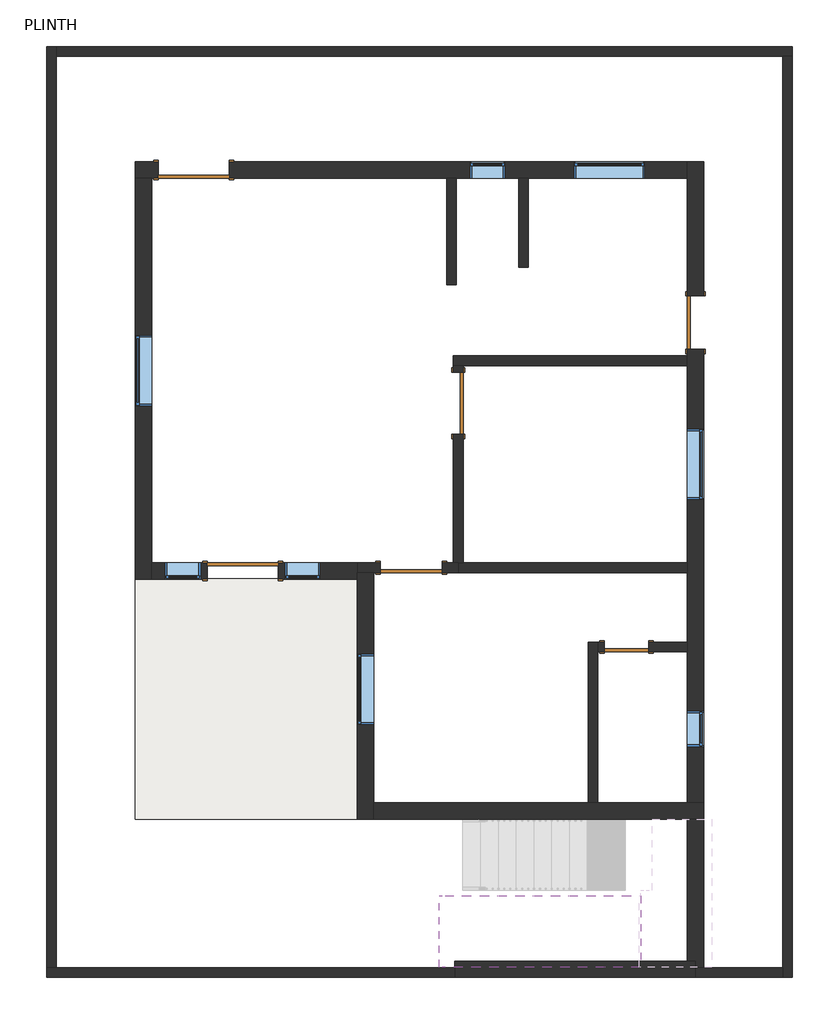
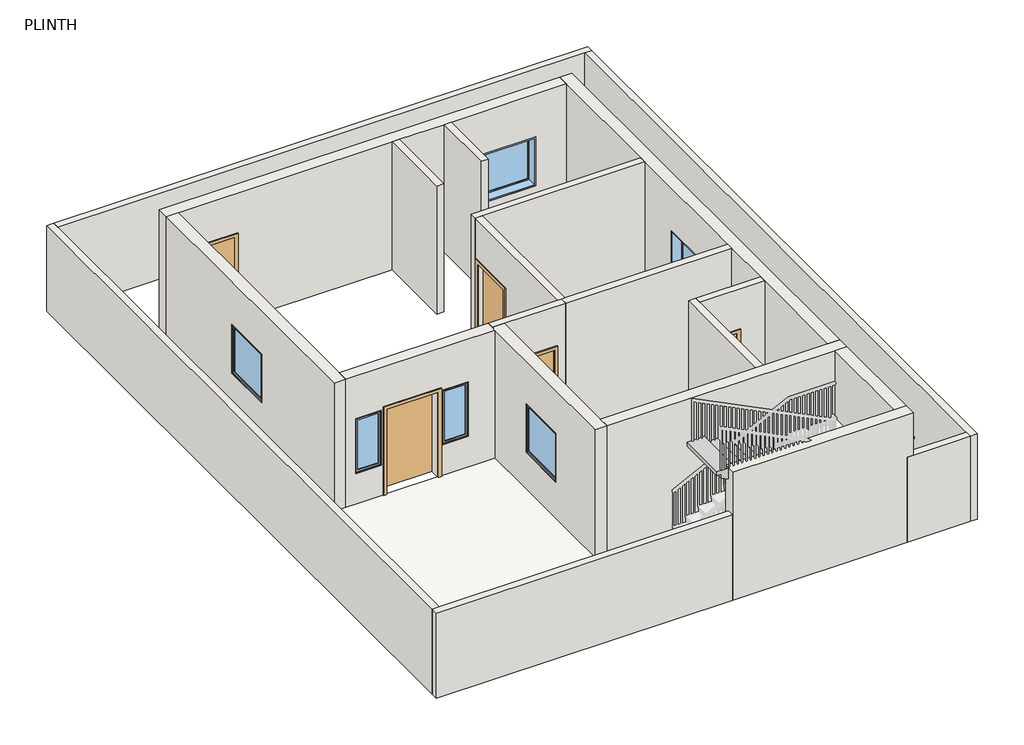
# One storey, part 1 of 3: 21 walls, 8 windows, 6 doors, 1 slab, 1 stair flight.
"""IFC4 building model written with IfcOpenShell, lengths in millimetres."""

from ifc_helpers import new_model, si_unit, frame, origin, origin_with_axes, place, context, project, spatial, polyline, outline, extrude, faceted_brep, transform, mapped, element, save
from components import door_9181f8a1, door_11d56761, door_bd8f54db, single_flush_3_x7_4f727f60, single_flush_4_x7_4e2c9459, single_flush_4_x7_d8936398, fixed_2_x2_ad5176ef, fixed_2_x4_5_07468de1, fixed_4_x4_67ff7140

model = new_model("IFC4")

# Units and contexts
model_context = context("Model", 3, world=origin())
ifc_project = project(units=[si_unit("LENGTHUNIT", "METRE", prefix="MILLI")], contexts=[model_context])

# Site, building, storey
site = spatial("IfcSite", under=ifc_project)
building = spatial("IfcBuilding", under=site)
storey = spatial("IfcBuildingStorey", under=building, Name="PLINTH", Elevation=0.0)

# Doors
placement = place(None, origin())
door_shape = door_9181f8a1(model_context)
element("IfcDoor", 1, ObjectType="Single-Flush : 2'6\"X7' 2", at=placement, inside=storey, context=model_context, shape_type="MappedRepresentation", body=[
    mapped(door_shape, transform((-10460.62252, 168.0193844, 0.0), x_axis=(-1.0, 0.0, 0.0), y_axis=(0.0, -1.0, 0.0), z_axis=(0.0, 0.0, 1.0))),
])
door_2_shape = door_11d56761(model_context)
element("IfcDoor", 2, ObjectType="Single-Flush : 3'6\"X7'", at=placement, inside=storey, context=model_context, shape_type="MappedRepresentation", body=[
    mapped(door_2_shape, transform((-14155.62252, 1526.2193844, 0.0), x_axis=(-1.0, 0.0, 0.0), y_axis=(0.0, -1.0, 0.0), z_axis=(0.0, 0.0, 1.0))),
])
door_3_shape = door_bd8f54db(model_context)
element("IfcDoor", 3, ObjectType="Single-Flush : 3'6\"X7'", at=placement, inside=storey, context=model_context, shape_type="MappedRepresentation", body=[
    mapped(door_3_shape, transform((-13348.82252, 4348.8193844, 0.0), x_axis=(0.0, 1.0, 0.0), y_axis=(-1.0, 0.0, 0.0), z_axis=(0.0, 0.0, 1.0))),
])
single_flush_3_x7_shape = single_flush_3_x7_4f727f60(model_context)
element("IfcDoor", 4, ObjectType="Single-Flush : 3'X7'", at=placement, inside=storey, context=model_context, shape_type="MappedRepresentation", body=[
    mapped(single_flush_3_x7_shape, transform((-9278.12252, 5733.8193844, 0.0), x_axis=(0.0, -1.0, 0.0), y_axis=(1.0, 0.0, 0.0), z_axis=(0.0, 0.0, 1.0))),
])
single_flush_4_x7_shape = single_flush_4_x7_4e2c9459(model_context)
element("IfcDoor", 5, ObjectType="Single-Flush : 4'X7'", at=placement, inside=storey, context=model_context, shape_type="MappedRepresentation", body=[
    mapped(single_flush_4_x7_shape, transform((-17886.62252, 8350.7193844, 0.0), x_axis=(-1.0, 0.0, 0.0), y_axis=(0.0, -1.0, 0.0), z_axis=(0.0, 0.0, 1.0))),
])
single_flush_4_x7_2_shape = single_flush_4_x7_d8936398(model_context)
element("IfcDoor", 6, ObjectType="Single-Flush : 4'X7'", at=placement, inside=storey, context=model_context, shape_type="MappedRepresentation", body=[
    mapped(single_flush_4_x7_2_shape, transform((-17048.42252, 1468.7193844, 0.0), x_axis=(-1.0, 0.0, 0.0), y_axis=(0.0, -1.0, 0.0), z_axis=(0.0, 0.0, 1.0))),
])

# Slab
element("IfcSlab", 7, ObjectType="Generic - 12\"", at=placement, inside=storey, context=model_context, shape_type="SweptSolid", body=[
    extrude(outline(polyline([(-15084.12252, 1341.7193844), (-15084.12252, -2786.4806156), (-18891.32252, -2786.4806156), (-18891.32252, 1341.7193844), (-15084.12252, 1341.7193844)])), frame((0.0, 0.0, -609.6), z_axis=(0.0, 0.0, 1.0), x_axis=(1.0, 0.0, 0.0)), (0.0, 0.0, 1.0), 609.6),
])

# Stair flight
element("IfcStairFlight", 8, ObjectType="3/4\" Nosing 6 1/2\" Depth", at=placement, inside=storey, context=model_context, shape_type="Brep", body=[
    faceted_brep([(-10219.32252, -4107.2806156, 1676.4), (-10219.32252, -5326.4806156, 1676.4), (-10238.37252, -5326.4806156, 1524.0), (-10238.37252, -4107.2806156, 1524.0), (-10543.17252, -4107.2806156, 1676.4), (-10543.17252, -5326.4806156, 1676.4), (-10543.17252, -5326.4806156, 1491.8125885), (-10238.37252, -5326.4806156, 1339.4125885), (-10238.37252, -4107.2806156, 1339.4125885), (-10543.17252, -4107.2806156, 1491.8125885), (-10524.12252, -5326.4806156, 1828.8), (-10524.12252, -4107.2806156, 1828.8), (-10847.97252, -4107.2806156, 1828.8), (-10847.97252, -5326.4806156, 1828.8), (-10847.97252, -5326.4806156, 1644.2125885), (-10847.97252, -4107.2806156, 1644.2125885), (-10828.92252, -5326.4806156, 1981.2), (-10828.92252, -4107.2806156, 1981.2), (-11152.77252, -4107.2806156, 1981.2), (-11152.77252, -5326.4806156, 1981.2), (-11152.77252, -5326.4806156, 1796.6125885), (-11152.77252, -4107.2806156, 1796.6125885), (-11133.72252, -5326.4806156, 2133.6), (-11133.72252, -4107.2806156, 2133.6), (-11457.57252, -4107.2806156, 2133.6), (-11457.57252, -5326.4806156, 2133.6), (-11457.57252, -5326.4806156, 1949.0125885), (-11457.57252, -4107.2806156, 1949.0125885), (-11438.52252, -5326.4806156, 2286.0), (-11438.52252, -4107.2806156, 2286.0), (-11762.37252, -4107.2806156, 2286.0), (-11762.37252, -5326.4806156, 2286.0), (-11762.37252, -5326.4806156, 2101.4125885), (-11762.37252, -4107.2806156, 2101.4125885), (-11743.32252, -5326.4806156, 2438.4), (-11743.32252, -4107.2806156, 2438.4), (-12067.17252, -4107.2806156, 2438.4), (-12067.17252, -5326.4806156, 2438.4), (-12067.17252, -5326.4806156, 2253.8125885), (-12067.17252, -4107.2806156, 2253.8125885), (-12048.12252, -5326.4806156, 2590.8), (-12048.12252, -4107.2806156, 2590.8), (-12371.97252, -4107.2806156, 2590.8), (-12371.97252, -5326.4806156, 2590.8), (-12371.97252, -5326.4806156, 2406.2125885), (-12371.97252, -4107.2806156, 2406.2125885), (-12352.92252, -5326.4806156, 2743.2), (-12352.92252, -4107.2806156, 2743.2), (-12676.77252, -4107.2806156, 2743.2), (-12676.77252, -5326.4806156, 2743.2), (-12676.77252, -5326.4806156, 2558.6125885), (-12676.77252, -4107.2806156, 2558.6125885), (-12657.72252, -5326.4806156, 2895.6), (-12657.72252, -4107.2806156, 2895.6), (-12981.57252, -4107.2806156, 2895.6), (-12981.57252, -5326.4806156, 2895.6), (-12981.57252, -5326.4806156, 2711.0125885), (-12981.57252, -4107.2806156, 2711.0125885), (-12962.52252, -5326.4806156, 3048.0), (-12962.52252, -4107.2806156, 3048.0), (-13286.37252, -4107.2806156, 3048.0), (-13286.37252, -5326.4806156, 3048.0), (-13286.37252, -5326.4806156, 2863.4125885), (-13286.37252, -4107.2806156, 2863.4125885), (-13267.32252, -5326.4806156, 3200.4), (-13267.32252, -4107.2806156, 3200.4), (-13673.72252, -4107.2806156, 3200.4), (-13673.72252, -5326.4806156, 3200.4), (-13673.72252, -5326.4806156, 3098.8), (-13572.12252, -5326.4806156, 3098.8), (-13572.12252, -5326.4806156, 3006.2875885), (-13572.12252, -4107.2806156, 3006.2875885), (-13572.12252, -4107.2806156, 3098.8), (-13673.72252, -4107.2806156, 3098.8)], [[[0, 1, 2, 3]], [[1, 0, 4, 5]], [[1, 5, 6, 7, 2]], [[3, 2, 7, 8]], [[4, 0, 3, 8, 9]], [[10, 11, 12, 13]], [[10, 13, 14, 6, 5]], [[12, 11, 4, 9, 15]], [[11, 10, 5, 4]], [[16, 17, 18, 19]], [[16, 19, 20, 14, 13]], [[18, 17, 12, 15, 21]], [[17, 16, 13, 12]], [[22, 23, 24, 25]], [[22, 25, 26, 20, 19]], [[24, 23, 18, 21, 27]], [[23, 22, 19, 18]], [[28, 29, 30, 31]], [[28, 31, 32, 26, 25]], [[30, 29, 24, 27, 33]], [[29, 28, 25, 24]], [[34, 35, 36, 37]], [[34, 37, 38, 32, 31]], [[36, 35, 30, 33, 39]], [[35, 34, 31, 30]], [[40, 41, 42, 43]], [[40, 43, 44, 38, 37]], [[42, 41, 36, 39, 45]], [[41, 40, 37, 36]], [[46, 47, 48, 49]], [[46, 49, 50, 44, 43]], [[48, 47, 42, 45, 51]], [[47, 46, 43, 42]], [[52, 53, 54, 55]], [[52, 55, 56, 50, 49]], [[54, 53, 48, 51, 57]], [[53, 52, 49, 48]], [[58, 59, 60, 61]], [[58, 61, 62, 56, 55]], [[60, 59, 54, 57, 63]], [[59, 58, 55, 54]], [[64, 65, 66, 67]], [[64, 67, 68, 69, 70, 62, 61]], [[66, 65, 60, 63, 71, 72, 73]], [[71, 70, 69, 72]], [[65, 64, 61, 60]], [[7, 6, 14, 20, 26, 32, 38, 44, 50, 56, 62, 70, 71, 63, 57, 51, 45, 39, 33, 27, 21, 15, 9, 8]], [[73, 72, 69, 68]], [[73, 68, 67, 66]]]),
])

# Walls
element("IfcWall", 9, ObjectType="4.5\" WALL", at=placement, inside=storey, context=model_context, shape_type="Brep", body=[
    faceted_brep([(-13431.72252, 4996.5193844, 0.0), (-13265.92252, 4996.5193844, 0.0), (-9418.52252, 4996.5193844, 0.0), (-9418.52252, 4996.5193844, 3200.4), (-13265.92252, 4996.5193844, 3200.4), (-13431.72252, 4996.5193844, 3200.4), (-13431.72252, 5162.3193844, 0.0), (-13431.72252, 5162.3193844, 3200.4), (-9418.52252, 5162.3193844, 3200.4), (-9418.52252, 5162.3193844, 0.0)], [[[0, 1, 2, 3, 4, 5]], [[6, 7, 8, 9]], [[2, 1, 0, 6, 9]], [[5, 4, 3, 8, 7]], [[3, 2, 9, 8]], [[0, 5, 7, 6]]]),
])
element("IfcWall", 10, ObjectType="4.5\" WALL", at=placement, inside=storey, context=model_context, shape_type="SweptSolid", body=[
    extrude(outline(polyline([(-13546.72252, 6381.5193844), (-13546.72252, 8210.3193844), (-13380.92252, 8210.3193844), (-13380.92252, 6381.5193844), (-13546.72252, 6381.5193844)])), origin_with_axes(), (0.0, 0.0, 1.0), 3200.4),
])
element("IfcWall", 11, ObjectType="4.5\" WALL", at=placement, inside=storey, context=model_context, shape_type="Brep", body=[
    faceted_brep([(-9418.52252, 1609.1193844, 0.0), (-13265.92252, 1609.1193844, 0.0), (-13348.82252, 1609.1193844, 0.0), (-13348.82252, 1609.1193844, 3200.4), (-13265.92252, 1609.1193844, 3200.4), (-9418.52252, 1609.1193844, 3200.4), (-9418.52252, 1443.3193844, 0.0), (-9418.52252, 1443.3193844, 3200.4), (-13348.82252, 1443.3193844, 3200.4), (-13348.82252, 1443.3193844, 0.0)], [[[0, 1, 2, 3, 4, 5]], [[6, 7, 8, 9]], [[2, 1, 0, 6, 9]], [[3, 2, 9, 8]], [[5, 4, 3, 8, 7]], [[0, 5, 7, 6]]]),
])
element("IfcWall", 12, ObjectType="4.5\" WALL", at=placement, inside=storey, context=model_context, shape_type="SweptSolid", body=[
    extrude(outline(polyline([(-12314.12252, 6686.3193844), (-12314.12252, 8210.3193844), (-12148.32252, 8210.3193844), (-12148.32252, 6686.3193844), (-12314.12252, 6686.3193844)])), origin_with_axes(), (0.0, 0.0, 1.0), 3200.4),
])
element("IfcWall", 13, ObjectType="4.5\" WALL", at=placement, inside=storey, context=model_context, shape_type="Brep", body=[
    faceted_brep([(-14689.02252, 1609.1193844, 2133.6), (-14689.02252, 1609.1193844, 0.0), (-15084.12252, 1609.1193844, 0.0), (-15084.12252, 1609.1193844, 3200.4), (-13431.72252, 1609.1193844, 3200.4), (-13348.82252, 1609.1193844, 3200.4), (-13348.82252, 1609.1193844, 0.0), (-13431.72252, 1609.1193844, 0.0), (-13622.22252, 1609.1193844, 0.0), (-13622.22252, 1609.1193844, 2133.6), (-15084.12252, 1443.3193844, 0.0), (-14803.32252, 1443.3193844, 0.0), (-14689.02252, 1443.3193844, 0.0), (-14689.02252, 1443.3193844, 2133.6), (-13622.22252, 1443.3193844, 2133.6), (-13622.22252, 1443.3193844, 0.0), (-13348.82252, 1443.3193844, 0.0), (-13348.82252, 1443.3193844, 3200.4), (-14803.32252, 1443.3193844, 3200.4), (-15084.12252, 1443.3193844, 3200.4)], [[[0, 1, 2, 3, 4, 5, 6, 7, 8, 9]], [[10, 11, 12, 13, 14, 15, 16, 17, 18, 19]], [[2, 1, 12, 11, 10]], [[8, 7, 6, 16, 15]], [[5, 4, 3, 19, 18, 17]], [[6, 5, 17, 16]], [[3, 2, 10, 19]], [[13, 12, 1, 0]], [[14, 13, 0, 9]], [[15, 14, 9, 8]]]),
])
element("IfcWall", 14, ObjectType="4.5\" WALL", at=placement, inside=storey, context=model_context, shape_type="Brep", body=[
    faceted_brep([(-13431.72252, 1609.1193844, 3200.4), (-13431.72252, 4996.5193844, 3200.4), (-13431.72252, 4996.5193844, 0.0), (-13431.72252, 4882.2193844, 0.0), (-13431.72252, 4882.2193844, 2133.6), (-13431.72252, 3815.4193844, 2133.6), (-13431.72252, 3815.4193844, 0.0), (-13431.72252, 1609.1193844, 0.0), (-13265.92252, 4996.5193844, 3200.4), (-13265.92252, 1609.1193844, 3200.4), (-13265.92252, 1609.1193844, 0.0), (-13265.92252, 3815.4193844, 0.0), (-13265.92252, 3815.4193844, 2133.6), (-13265.92252, 4882.2193844, 2133.6), (-13265.92252, 4882.2193844, 0.0), (-13265.92252, 4996.5193844, 0.0), (-13348.82252, 1609.1193844, 0.0), (-13348.82252, 1609.1193844, 3200.4)], [[[0, 1, 2, 3, 4, 5, 6, 7]], [[8, 9, 10, 11, 12, 13, 14, 15]], [[2, 15, 14, 3]], [[10, 16, 7, 6, 11]], [[1, 0, 17, 9, 8]], [[2, 1, 8, 15]], [[0, 7, 16, 10, 9, 17]], [[13, 4, 3, 14]], [[4, 13, 12, 5]], [[5, 12, 11, 6]]]),
])
element("IfcWall", 15, ObjectType="4.5\" WALL", at=placement, inside=storey, context=model_context, shape_type="Brep", body=[
    faceted_brep([(-11121.72252, 250.9193844, 0.0), (-11121.72252, -2505.6806156, 0.0), (-11121.72252, -2505.6806156, 3200.4), (-11121.72252, 250.9193844, 3200.4), (-10955.92252, 250.9193844, 0.0), (-10955.92252, 250.9193844, 3200.4), (-10955.92252, 85.1193844, 3200.4), (-10955.92252, -2505.6806156, 3200.4), (-10955.92252, -2505.6806156, 0.0), (-10955.92252, 85.1193844, 0.0)], [[[0, 1, 2, 3]], [[4, 5, 6, 7, 8, 9]], [[1, 0, 4, 9, 8]], [[3, 2, 7, 6, 5]], [[0, 3, 5, 4]], [[2, 1, 8, 7]]]),
])
element("IfcWall", 16, ObjectType="4.5\" WALL", at=placement, inside=storey, context=model_context, shape_type="SweptSolid", body=[
    extrude(outline(polyline([(3200.4, -9418.52252), (3200.4, -10955.92252), (0.0, -10955.92252), (0.0, -10841.62252), (2133.6, -10841.62252), (2133.6, -10079.62252), (0.0, -10079.62252), (0.0, -9418.52252), (3200.4, -9418.52252)])), frame((0.0, 85.1193844, 0.0), z_axis=(0.0, 1.0, 0.0), x_axis=(0.0, 0.0, 1.0)), (0.0, 0.0, 1.0), 165.8),
])
element("IfcWall", 17, ObjectType="9\" WALL", at=placement, inside=storey, context=model_context, shape_type="Brep", body=[
    faceted_brep([(-18891.32252, 8210.3193844, 0.0), (-18610.52252, 8210.3193844, 0.0), (-18496.22252, 8210.3193844, 0.0), (-18496.22252, 8210.3193844, 2133.6), (-17277.02252, 8210.3193844, 2133.6), (-17277.02252, 8210.3193844, 0.0), (-13546.72252, 8210.3193844, 0.0), (-13380.92252, 8210.3193844, 0.0), (-12314.12252, 8210.3193844, 0.0), (-12148.32252, 8210.3193844, 0.0), (-9418.52252, 8210.3193844, 0.0), (-9418.52252, 8210.3193844, 3200.4), (-12148.32252, 8210.3193844, 3200.4), (-12314.12252, 8210.3193844, 3200.4), (-13380.92252, 8210.3193844, 3200.4), (-13546.72252, 8210.3193844, 3200.4), (-18610.52252, 8210.3193844, 3200.4), (-18891.32252, 8210.3193844, 3200.4), (-10145.07252, 8210.3193844, 2133.6), (-10145.07252, 8210.3193844, 914.4), (-11364.27252, 8210.3193844, 914.4), (-11364.27252, 8210.3193844, 2133.6), (-12542.72252, 8210.3193844, 1524.0), (-12542.72252, 8210.3193844, 914.4), (-13152.32252, 8210.3193844, 914.4), (-13152.32252, 8210.3193844, 1524.0), (-18496.22252, 8491.1193844, 2133.6), (-18496.22252, 8491.1193844, 0.0), (-18891.32252, 8491.1193844, 0.0), (-18891.32252, 8491.1193844, 3200.4), (-9418.52252, 8491.1193844, 3200.4), (-9418.52252, 8491.1193844, 0.0), (-17277.02252, 8491.1193844, 0.0), (-17277.02252, 8491.1193844, 2133.6), (-10145.07252, 8491.1193844, 2133.6), (-11364.27252, 8491.1193844, 2133.6), (-11364.27252, 8491.1193844, 914.4), (-10145.07252, 8491.1193844, 914.4), (-12542.72252, 8491.1193844, 1524.0), (-13152.32252, 8491.1193844, 1524.0), (-13152.32252, 8491.1193844, 914.4), (-12542.72252, 8491.1193844, 914.4)], [[[0, 1, 2, 3, 4, 5, 6, 7, 8, 9, 10, 11, 12, 13, 14, 15, 16, 17], [18, 19, 20, 21], [22, 23, 24, 25]], [[26, 27, 28, 29, 30, 31, 32, 33], [34, 35, 36, 37], [38, 39, 40, 41]], [[32, 31, 10, 9, 8, 7, 6, 5]], [[28, 27, 2, 1, 0]], [[17, 16, 15, 14, 13, 12, 11, 30, 29]], [[0, 17, 29, 28]], [[11, 10, 31, 30]], [[3, 2, 27, 26]], [[4, 3, 26, 33]], [[5, 4, 33, 32]], [[19, 18, 34, 37]], [[20, 19, 37, 36]], [[21, 20, 36, 35]], [[18, 21, 35, 34]], [[23, 22, 38, 41]], [[24, 23, 41, 40]], [[25, 24, 40, 39]], [[22, 25, 39, 38]]]),
])
element("IfcWall", 18, ObjectType="9\" WALL", at=placement, inside=storey, context=model_context, shape_type="Brep", body=[
    faceted_brep([(-18610.52252, 1328.3193844, 0.0), (-18610.52252, 1609.1193844, 0.0), (-18610.52252, 8210.3193844, 0.0), (-18610.52252, 8210.3193844, 3200.4), (-18610.52252, 1609.1193844, 3200.4), (-18610.52252, 1328.3193844, 3200.4), (-18610.52252, 5519.3193844, 2133.6), (-18610.52252, 5519.3193844, 914.4), (-18610.52252, 4300.1193844, 914.4), (-18610.52252, 4300.1193844, 2133.6), (-18891.32252, 1328.3193844, 0.0), (-18891.32252, 1328.3193844, 3200.4), (-18891.32252, 8210.3193844, 3200.4), (-18891.32252, 8210.3193844, 0.0), (-18891.32252, 5519.3193844, 2133.6), (-18891.32252, 4300.1193844, 2133.6), (-18891.32252, 4300.1193844, 914.4), (-18891.32252, 5519.3193844, 914.4)], [[[0, 1, 2, 3, 4, 5], [6, 7, 8, 9]], [[10, 11, 12, 13], [14, 15, 16, 17]], [[2, 1, 0, 10, 13]], [[5, 4, 3, 12, 11]], [[3, 2, 13, 12]], [[0, 5, 11, 10]], [[7, 6, 14, 17]], [[8, 7, 17, 16]], [[9, 8, 16, 15]], [[6, 9, 15, 14]]]),
])
element("IfcWall", 19, ObjectType="9\" WALL", at=placement, inside=storey, context=model_context, shape_type="Brep", body=[
    faceted_brep([(-9137.72252, -2505.6806156, 0.0), (-9418.52252, -2505.6806156, 0.0), (-10955.92252, -2505.6806156, 0.0), (-11121.72252, -2505.6806156, 0.0), (-14803.32252, -2505.6806156, 0.0), (-14803.32252, -2505.6806156, 3200.4), (-11121.72252, -2505.6806156, 3200.4), (-10955.92252, -2505.6806156, 3200.4), (-9418.52252, -2505.6806156, 3200.4), (-9137.72252, -2505.6806156, 3200.4), (-9137.72252, -2786.4806156, 0.0), (-9137.72252, -2786.4806156, 3200.4), (-9418.52252, -2786.4806156, 3200.4), (-14803.32252, -2786.4806156, 3200.4), (-14803.32252, -2786.4806156, 0.0), (-9418.52252, -2786.4806156, 0.0)], [[[0, 1, 2, 3, 4, 5, 6, 7, 8, 9]], [[10, 11, 12, 13, 14, 15]], [[4, 3, 2, 1, 0, 10, 15, 14]], [[9, 8, 7, 6, 5, 13, 12, 11]], [[0, 9, 11, 10]], [[5, 4, 14, 13]]]),
])
element("IfcWall", 20, ObjectType="9\" WALL", at=placement, inside=storey, context=model_context, shape_type="Brep", body=[
    faceted_brep([(-9418.52252, 5276.6193844, 2133.6), (-9418.52252, 5276.6193844, 0.0), (-9418.52252, 5162.3193844, 0.0), (-9418.52252, 4996.5193844, 0.0), (-9418.52252, 1609.1193844, 0.0), (-9418.52252, 1443.3193844, 0.0), (-9418.52252, 250.9193844, 0.0), (-9418.52252, 85.1193844, 0.0), (-9418.52252, -2505.6806156, 0.0), (-9418.52252, -2505.6806156, 3200.4), (-9418.52252, 85.1193844, 3200.4), (-9418.52252, 250.9193844, 3200.4), (-9418.52252, 1443.3193844, 3200.4), (-9418.52252, 1609.1193844, 3200.4), (-9418.52252, 4996.5193844, 3200.4), (-9418.52252, 5162.3193844, 3200.4), (-9418.52252, 8210.3193844, 3200.4), (-9418.52252, 8491.1193844, 3200.4), (-9418.52252, 8491.1193844, 0.0), (-9418.52252, 8210.3193844, 0.0), (-9418.52252, 6191.0193844, 0.0), (-9418.52252, 6191.0193844, 2133.6), (-9418.52252, 2693.2193844, 2133.6), (-9418.52252, 2693.2193844, 914.4), (-9418.52252, 3912.4193844, 914.4), (-9418.52252, 3912.4193844, 2133.6), (-9418.52252, -1543.8306156, 1524.0), (-9418.52252, -1543.8306156, 914.4), (-9418.52252, -934.2306156, 914.4), (-9418.52252, -934.2306156, 1524.0), (-9137.72252, -2505.6806156, 0.0), (-9137.72252, 5276.6193844, 0.0), (-9137.72252, 5276.6193844, 2133.6), (-9137.72252, 6191.0193844, 2133.6), (-9137.72252, 6191.0193844, 0.0), (-9137.72252, 8491.1193844, 0.0), (-9137.72252, 8491.1193844, 3200.4), (-9137.72252, -2505.6806156, 3200.4), (-9137.72252, 2693.2193844, 2133.6), (-9137.72252, 3912.4193844, 2133.6), (-9137.72252, 3912.4193844, 914.4), (-9137.72252, 2693.2193844, 914.4), (-9137.72252, -1543.8306156, 1524.0), (-9137.72252, -934.2306156, 1524.0), (-9137.72252, -934.2306156, 914.4), (-9137.72252, -1543.8306156, 914.4)], [[[0, 1, 2, 3, 4, 5, 6, 7, 8, 9, 10, 11, 12, 13, 14, 15, 16, 17, 18, 19, 20, 21], [22, 23, 24, 25], [26, 27, 28, 29]], [[30, 31, 32, 33, 34, 35, 36, 37], [38, 39, 40, 41], [42, 43, 44, 45]], [[20, 19, 18, 35, 34]], [[8, 7, 6, 5, 4, 3, 2, 1, 31, 30]], [[17, 16, 15, 14, 13, 12, 11, 10, 9, 37, 36]], [[18, 17, 36, 35]], [[9, 8, 30, 37]], [[23, 22, 38, 41]], [[24, 23, 41, 40]], [[25, 24, 40, 39]], [[22, 25, 39, 38]], [[32, 31, 1, 0]], [[33, 32, 0, 21]], [[34, 33, 21, 20]], [[27, 26, 42, 45]], [[28, 27, 45, 44]], [[29, 28, 44, 43]], [[26, 29, 43, 42]]]),
])
element("IfcWall", 21, ObjectType="9\" WALL", at=placement, inside=storey, context=model_context, shape_type="Brep", body=[
    faceted_brep([(-15084.12252, 1443.3193844, 0.0), (-15084.12252, 1328.3193844, 0.0), (-15084.12252, -2786.4806156, 0.0), (-15084.12252, -2786.4806156, 3200.4), (-15084.12252, 1328.3193844, 3200.4), (-15084.12252, 1443.3193844, 3200.4), (-15084.12252, 49.6693844, 2133.6), (-15084.12252, -1169.5306156, 2133.6), (-15084.12252, -1169.5306156, 914.4), (-15084.12252, 49.6693844, 914.4), (-14803.32252, 1443.3193844, 0.0), (-14803.32252, 1443.3193844, 3200.4), (-14803.32252, -2505.6806156, 3200.4), (-14803.32252, -2786.4806156, 3200.4), (-14803.32252, -2786.4806156, 0.0), (-14803.32252, -2505.6806156, 0.0), (-14803.32252, 49.6693844, 2133.6), (-14803.32252, 49.6693844, 914.4), (-14803.32252, -1169.5306156, 914.4), (-14803.32252, -1169.5306156, 2133.6)], [[[0, 1, 2, 3, 4, 5], [6, 7, 8, 9]], [[10, 11, 12, 13, 14, 15], [16, 17, 18, 19]], [[2, 1, 0, 10, 15, 14]], [[5, 4, 3, 13, 12, 11]], [[3, 2, 14, 13]], [[0, 5, 11, 10]], [[17, 16, 6, 9]], [[18, 17, 9, 8]], [[19, 18, 8, 7]], [[16, 19, 7, 6]]]),
])
element("IfcWall", 22, ObjectType="9\" WALL", at=placement, inside=storey, context=model_context, shape_type="Brep", body=[
    faceted_brep([(-17658.02252, 1609.1193844, 2133.6), (-17658.02252, 1609.1193844, 0.0), (-18610.52252, 1609.1193844, 0.0), (-18610.52252, 1609.1193844, 3200.4), (-15084.12252, 1609.1193844, 3200.4), (-15084.12252, 1609.1193844, 0.0), (-16438.82252, 1609.1193844, 0.0), (-16438.82252, 1609.1193844, 2133.6), (-16322.831064, 1609.1193844, 2133.6), (-16322.831064, 1609.1193844, 762.0), (-15713.231064, 1609.1193844, 762.0), (-15713.231064, 1609.1193844, 2133.6), (-18381.92252, 1609.1193844, 2133.6), (-18381.92252, 1609.1193844, 762.0), (-17772.32252, 1609.1193844, 762.0), (-17772.32252, 1609.1193844, 2133.6), (-18610.52252, 1328.3193844, 0.0), (-17658.02252, 1328.3193844, 0.0), (-17658.02252, 1328.3193844, 2133.6), (-16438.82252, 1328.3193844, 2133.6), (-16438.82252, 1328.3193844, 0.0), (-15084.12252, 1328.3193844, 0.0), (-15084.12252, 1328.3193844, 3200.4), (-18610.52252, 1328.3193844, 3200.4), (-16322.831064, 1328.3193844, 2133.6), (-15713.231064, 1328.3193844, 2133.6), (-15713.231064, 1328.3193844, 762.0), (-16322.831064, 1328.3193844, 762.0), (-18381.92252, 1328.3193844, 2133.6), (-17772.32252, 1328.3193844, 2133.6), (-17772.32252, 1328.3193844, 762.0), (-18381.92252, 1328.3193844, 762.0), (-15084.12252, 1443.3193844, 0.0), (-15084.12252, 1443.3193844, 3200.4)], [[[0, 1, 2, 3, 4, 5, 6, 7], [8, 9, 10, 11], [12, 13, 14, 15]], [[16, 17, 18, 19, 20, 21, 22, 23], [24, 25, 26, 27], [28, 29, 30, 31]], [[6, 5, 32, 21, 20]], [[2, 1, 17, 16]], [[4, 3, 23, 22, 33]], [[3, 2, 16, 23]], [[5, 4, 33, 22, 21, 32]], [[18, 17, 1, 0]], [[19, 18, 0, 7]], [[20, 19, 7, 6]], [[9, 8, 24, 27]], [[10, 9, 27, 26]], [[11, 10, 26, 25]], [[8, 11, 25, 24]], [[13, 12, 28, 31]], [[14, 13, 31, 30]], [[15, 14, 30, 29]], [[12, 15, 29, 28]]]),
])
element("IfcWall", 23, ObjectType="9\" WALL", at=placement, inside=storey, context=model_context, shape_type="Brep", body=[
    faceted_brep([(-9278.12252, -5224.8806156, 0.0), (-9418.52252, -5224.8806156, 0.0), (-13404.92252, -5224.8806156, 0.0), (-13404.92252, -5224.8806156, 3200.4), (-9418.52252, -5224.8806156, 3200.4), (-9137.72252, -5224.8806156, 3200.4), (-9137.72252, -5224.8806156, 2133.6), (-9278.12252, -5224.8806156, 2133.6), (-9278.12252, -5505.6806156, 0.0), (-9278.12252, -5505.6806156, 2133.6), (-9137.72252, -5505.6806156, 2133.6), (-9137.72252, -5505.6806156, 3200.4), (-13404.92252, -5505.6806156, 3200.4), (-13404.92252, -5505.6806156, 0.0), (-9278.12252, -5339.8806156, 0.0), (-13404.92252, -5339.8806156, 0.0), (-9278.12252, -5339.8806156, 2133.6), (-9137.72252, -5339.8806156, 2133.6)], [[[0, 1, 2, 3, 4, 5, 6, 7]], [[8, 9, 10, 11, 12, 13]], [[2, 1, 0, 14, 8, 13, 15]], [[3, 2, 15, 13, 12]], [[5, 4, 3, 12, 11]], [[0, 7, 16, 9, 8, 14]], [[6, 17, 10, 9, 16, 7]], [[6, 5, 11, 10, 17]]]),
])
element("IfcWall", 24, ObjectType="9\" WALL", at=placement, inside=storey, context=model_context, shape_type="Brep", body=[
    faceted_brep([(-9418.52252, -2786.4806156, 0.0), (-9418.52252, -5224.8806156, 0.0), (-9418.52252, -5224.8806156, 2133.6), (-9418.52252, -5224.8806156, 3200.4), (-9418.52252, -2786.4806156, 3200.4), (-9137.72252, -2786.4806156, 0.0), (-9137.72252, -2786.4806156, 3200.4), (-9137.72252, -5224.8806156, 3200.4), (-9137.72252, -5224.8806156, 2133.6), (-9137.72252, -5339.8806156, 2133.6), (-9137.72252, -5339.8806156, 0.0), (-9278.12252, -5339.8806156, 0.0), (-9278.12252, -5224.8806156, 0.0), (-9278.12252, -5224.8806156, 2133.6), (-9278.12252, -5339.8806156, 2133.6)], [[[0, 1, 2, 3, 4]], [[5, 6, 7, 8, 9, 10]], [[1, 0, 5, 10, 11, 12]], [[4, 3, 7, 6]], [[0, 4, 6, 5]], [[8, 13, 14, 9]], [[2, 1, 12, 13]], [[12, 11, 14, 13]], [[11, 10, 9, 14]], [[3, 2, 13, 8, 7]]]),
])
element("IfcWall", 25, ObjectType="COMPOUND WALL", at=placement, inside=storey, context=model_context, shape_type="Brep", body=[
    faceted_brep([(-13404.92252, -5339.8806156, 0.0), (-20249.52252, -5339.8806156, 0.0), (-20415.32252, -5339.8806156, 0.0), (-20415.32252, -5339.8806156, 2133.6), (-20249.52252, -5339.8806156, 2133.6), (-13404.92252, -5339.8806156, 2133.6), (-13404.92252, -5505.6806156, 0.0), (-13404.92252, -5505.6806156, 2133.6), (-20415.32252, -5505.6806156, 2133.6), (-20415.32252, -5505.6806156, 0.0)], [[[0, 1, 2, 3, 4, 5]], [[6, 7, 8, 9]], [[2, 1, 0, 6, 9]], [[5, 4, 3, 8, 7]], [[0, 5, 7, 6]], [[3, 2, 9, 8]]]),
])
element("IfcWall", 26, ObjectType="COMPOUND WALL", at=placement, inside=storey, context=model_context, shape_type="Brep", body=[
    faceted_brep([(-20249.52252, -5339.8806156, 0.0), (-20249.52252, 10306.5193844, 0.0), (-20249.52252, 10472.3193844, 0.0), (-20249.52252, 10472.3193844, 2133.6), (-20249.52252, 10306.5193844, 2133.6), (-20249.52252, -5339.8806156, 2133.6), (-20415.32252, -5339.8806156, 0.0), (-20415.32252, -5339.8806156, 2133.6), (-20415.32252, 10472.3193844, 2133.6), (-20415.32252, 10472.3193844, 0.0)], [[[0, 1, 2, 3, 4, 5]], [[6, 7, 8, 9]], [[2, 1, 0, 6, 9]], [[5, 4, 3, 8, 7]], [[0, 5, 7, 6]], [[3, 2, 9, 8]]]),
])
element("IfcWall", 27, ObjectType="COMPOUND WALL", at=placement, inside=storey, context=model_context, shape_type="Brep", body=[
    faceted_brep([(-20249.52252, 10306.5193844, 0.0), (-7779.52252, 10306.5193844, 0.0), (-7613.72252, 10306.5193844, 0.0), (-7613.72252, 10306.5193844, 2133.6), (-7779.52252, 10306.5193844, 2133.6), (-20249.52252, 10306.5193844, 2133.6), (-20249.52252, 10472.3193844, 0.0), (-20249.52252, 10472.3193844, 2133.6), (-7613.72252, 10472.3193844, 2133.6), (-7613.72252, 10472.3193844, 0.0)], [[[0, 1, 2, 3, 4, 5]], [[6, 7, 8, 9]], [[2, 1, 0, 6, 9]], [[5, 4, 3, 8, 7]], [[0, 5, 7, 6]], [[3, 2, 9, 8]]]),
])
element("IfcWall", 28, ObjectType="COMPOUND WALL", at=placement, inside=storey, context=model_context, shape_type="Brep", body=[
    faceted_brep([(-7779.52252, 10306.5193844, 0.0), (-7779.52252, -5339.8806156, 0.0), (-7779.52252, -5505.6806156, 0.0), (-7779.52252, -5505.6806156, 2133.6), (-7779.52252, -5339.8806156, 2133.6), (-7779.52252, 10306.5193844, 2133.6), (-7613.72252, 10306.5193844, 0.0), (-7613.72252, 10306.5193844, 2133.6), (-7613.72252, -5505.6806156, 2133.6), (-7613.72252, -5505.6806156, 0.0)], [[[0, 1, 2, 3, 4, 5]], [[6, 7, 8, 9]], [[2, 1, 0, 6, 9]], [[5, 4, 3, 8, 7]], [[0, 5, 7, 6]], [[3, 2, 9, 8]]]),
])
element("IfcWall", 29, ObjectType="COMPOUND WALL", at=placement, inside=storey, context=model_context, shape_type="Brep", body=[
    faceted_brep([(-7779.52252, -5339.8806156, 0.0), (-9137.72252, -5339.8806156, 0.0), (-9278.12252, -5339.8806156, 0.0), (-9278.12252, -5339.8806156, 2133.6), (-9137.72252, -5339.8806156, 2133.6), (-7779.52252, -5339.8806156, 2133.6), (-7779.52252, -5505.6806156, 0.0), (-7779.52252, -5505.6806156, 2133.6), (-9278.12252, -5505.6806156, 2133.6), (-9278.12252, -5505.6806156, 0.0)], [[[0, 1, 2, 3, 4, 5]], [[6, 7, 8, 9]], [[2, 1, 0, 6, 9]], [[3, 2, 9, 8]], [[5, 4, 3, 8, 7]], [[0, 5, 7, 6]]]),
])

# Windows
fixed_2_x2_shape = fixed_2_x2_ad5176ef(model_context)
element("IfcWindow", 30, ObjectType="Fixed : 2'X2'", at=placement, inside=storey, context=model_context, shape_type="MappedRepresentation", body=[
    mapped(fixed_2_x2_shape, transform((-9278.12252, -1277.1306156, 0.0), x_axis=(0.0, -1.0, 0.0), y_axis=(1.0, 0.0, 0.0), z_axis=(0.0, 0.0, 1.0))),
])
element("IfcWindow", 31, ObjectType="Fixed : 2'X2'", at=placement, inside=storey, context=model_context, shape_type="MappedRepresentation", body=[
    mapped(fixed_2_x2_shape, transform((-12809.42252, 8350.7193844, 0.0), x_axis=(1.0, 0.0, 0.0), y_axis=(0.0, 1.0, 0.0), z_axis=(0.0, 0.0, 1.0))),
])
fixed_2_x4_5_shape = fixed_2_x4_5_07468de1(model_context)
element("IfcWindow", 32, ObjectType="Fixed : 2'X4.5'", at=placement, inside=storey, context=model_context, shape_type="MappedRepresentation", body=[
    mapped(fixed_2_x4_5_shape, transform((-16056.131064, 1468.7193844, 0.0), x_axis=(-1.0, 0.0, 0.0), y_axis=(0.0, -1.0, 0.0), z_axis=(0.0, 0.0, 1.0))),
])
element("IfcWindow", 33, ObjectType="Fixed : 2'X4.5'", at=placement, inside=storey, context=model_context, shape_type="MappedRepresentation", body=[
    mapped(fixed_2_x4_5_shape, transform((-18115.22252, 1468.7193844, 0.0), x_axis=(-1.0, 0.0, 0.0), y_axis=(0.0, -1.0, 0.0), z_axis=(0.0, 0.0, 1.0))),
])
fixed_4_x4_shape = fixed_4_x4_67ff7140(model_context)
element("IfcWindow", 34, ObjectType="Fixed : 4'X4'", at=placement, inside=storey, context=model_context, shape_type="MappedRepresentation", body=[
    mapped(fixed_4_x4_shape, transform((-9278.12252, 3264.7193844, 0.0), x_axis=(0.0, -1.0, 0.0), y_axis=(1.0, 0.0, 0.0), z_axis=(0.0, 0.0, 1.0))),
])
element("IfcWindow", 35, ObjectType="Fixed : 4'X4'", at=placement, inside=storey, context=model_context, shape_type="MappedRepresentation", body=[
    mapped(fixed_4_x4_shape, transform((-14943.72252, -521.8306156, 0.0), x_axis=(0.0, 1.0, 0.0), y_axis=(-1.0, 0.0, 0.0), z_axis=(0.0, 0.0, 1.0))),
])
element("IfcWindow", 36, ObjectType="Fixed : 4'X4'", at=placement, inside=storey, context=model_context, shape_type="MappedRepresentation", body=[
    mapped(fixed_4_x4_shape, transform((-18750.92252, 4947.8193844, 0.0), x_axis=(0.0, 1.0, 0.0), y_axis=(-1.0, 0.0, 0.0), z_axis=(0.0, 0.0, 1.0))),
])
element("IfcWindow", 37, ObjectType="Fixed : 4'X4'", at=placement, inside=storey, context=model_context, shape_type="MappedRepresentation", body=[
    mapped(fixed_4_x4_shape, transform((-10716.57252, 8350.7193844, 0.0), x_axis=(1.0, 0.0, 0.0), y_axis=(0.0, 1.0, 0.0), z_axis=(0.0, 0.0, 1.0))),
])

save(model, "model.ifc")

# Revit data of these elements
# Type "Single-Flush : 2'6\"X7' 2"
#   Type Mark = "9"
#   Assembly Code = "C1020"
#   Thickness = 0' - 2"
#   Height = 7' - 0"
#   Trim Projection Ext = 0' - 1"
#   Trim Projection Int = 0' - 1"
#   Trim Width = 0' - 3"
#   Width = 2' - 6"
#   Door Material = Door - Panel
#   Frame Material = Door - Frame
#   Function = (empty or 0)
#   Wall Closure = (empty or 0)
# Type "Single-Flush : 3'6\"X7'"
#   Type Mark = "8"
#   Assembly Code = "C1020"
#   Thickness = 0' - 2"
#   Height = 7' - 0"
#   Trim Projection Ext = 0' - 1"
#   Trim Projection Int = 0' - 1"
#   Trim Width = 0' - 3"
#   Width = 3' - 6"
#   Door Material = Door - Panel
#   Frame Material = Door - Frame
#   Function = (empty or 0)
#   Wall Closure = (empty or 0)
# Type "Single-Flush : 3'X7'"
#   Type Mark = "10"
#   Assembly Code = "C1020"
#   Thickness = 0' - 2"
#   Height = 7' - 0"
#   Trim Projection Ext = 0' - 1"
#   Trim Projection Int = 0' - 1"
#   Trim Width = 0' - 3"
#   Width = 3' - 0"
#   Door Material = Door - Panel
#   Frame Material = Door - Frame
#   Function = (empty or 0)
#   Wall Closure = (empty or 0)
# Type "Single-Flush : 4'X7'"
#   Type Mark = "11"
#   Assembly Code = "C1020"
#   Thickness = 0' - 2"
#   Height = 7' - 0"
#   Trim Projection Ext = 0' - 1"
#   Trim Projection Int = 0' - 1"
#   Trim Width = 0' - 3"
#   Width = 4' - 0"
#   Door Material = Door - Panel
#   Frame Material = Door - Frame
#   Function = (empty or 0)
#   Wall Closure = (empty or 0)
# Type "Generic - 12\""
#   Assembly Code = "B1010"
#   Function = 0
#   Layers, outside or top first: 2' - 0" "Concrete, Cast-in-Place gray" (function 1)
# Type "4.5\" WALL"
#   Layers, outside or top first: 0' - 1" "PLASTER OUTER" (function 4); 0' - 4.52756" "Brick, Soldier Course" (function 1); 0' - 1" "PLASTER INNER" (function 5)
# Type "9\" WALL"
#   Layers, outside or top first: 0' - 1" "PLASTER OUTER" (function 4); 0' - 9.05512" "Brick, Common" (function 1); 0' - 1" "PLASTER INNER" (function 5)
# Type "COMPOUND WALL"
#   Layers, outside or top first: 0' - 1" "PLASTER OUTER" (function 4); 0' - 4.52756" "Brick, Soldier Course" (function 1); 0' - 1" "PLASTER INNER" (function 5)
# Type "Fixed : 2'X2'"
#   Type Mark = "11"
#   Assembly Code = "B2020100"
#   Height = 2' - 0"
#   Default Sill Height = 3' - 0"
#   Width = 2' - 0"
#   Window Inset = 0' - 0 3/4"
#   Glass Pane Material = Glass
#   Sash Material = Sash
#   Wall Closure = (empty or 0)
# Type "Fixed : 2'X4.5'"
#   Type Mark = "12"
#   Assembly Code = "B2020100"
#   Height = 4' - 6"
#   Default Sill Height = 2' - 6"
#   Width = 2' - 0"
#   Window Inset = 0' - 0 3/4"
#   Glass Pane Material = Glass
#   Sash Material = Sash
#   Wall Closure = (empty or 0)
# Type "Fixed : 4'X4'"
#   Type Mark = "10"
#   Assembly Code = "B2020100"
#   Height = 4' - 0"
#   Default Sill Height = 3' - 0"
#   Width = 4' - 0"
#   Window Inset = 0' - 0 3/4"
#   Glass Pane Material = Glass
#   Sash Material = Sash
#   Wall Closure = (empty or 0)
# Element 1 (IfcDoor, "Single-Flush : 2'6\"X7' 2")
#   Phase Created = New Construction
#   Materials on its faces: "Door - Frame", "Door - Panel"
# Elements 2, 3 (IfcDoor, "Single-Flush : 3'6\"X7'")
#   Phase Created = New Construction
#   Materials on its faces: "Door - Frame", "Door - Panel"
# Element 4 (IfcDoor, "Single-Flush : 3'X7'")
#   Phase Created = New Construction
#   Materials on its faces: "Door - Frame", "Door - Panel"
# Elements 5, 6 (IfcDoor, "Single-Flush : 4'X7'")
#   Phase Created = New Construction
#   Materials on its faces: "Door - Frame", "Door - Panel"
# Element 7 (IfcSlab, "Generic - 12\"")
#   Height Offset From Level = 0' - 0"
#   Phase Created = New Construction
#   Materials on its faces: "Concrete, Cast-in-Place gray"
# Element 8 (IfcStairFlight, "3/4\" Nosing 6 1/2\" Depth")
#   Phase Created = New Construction
#   Materials on its faces: "Concrete, Cast-in-Place gray"
# Elements 9, 10, 11, 12, 13, 14, 16 (IfcWall, "4.5\" WALL")
#   Top Offset = 0' - 0"
#   Base Offset = 0' - 0"
#   wall height = 10' - 6"
#   Phase Created = New Construction
#   Base Constraint = PLINTH
#   Top Constraint = GF
#   Materials on its faces: "Default Wall", "PLASTER INNER", "PLASTER OUTER"
# Element 15 (IfcWall, "4.5\" WALL")
#   Top Offset = 0' - 0"
#   Base Offset = 0' - 0"
#   wall height = 10' - 6"
#   Phase Created = New Construction
#   Base Constraint = PLINTH
#   Top Constraint = GF
#   Materials on its faces: "Default Wall", "PLASTER OUTER", "PLASTER INNER"
# Elements 17, 18, 19, 20, 21, 24 (IfcWall, "9\" WALL")
#   Top Offset = 0' - 0"
#   Base Offset = 0' - 0"
#   wall height = 10' - 6"
#   Phase Created = New Construction
#   Base Constraint = PLINTH
#   Top Constraint = GF
#   Materials on its faces: "Default Wall", "PLASTER OUTER", "PLASTER INNER"
# Elements 22, 23 (IfcWall, "9\" WALL")
#   Top Offset = 0' - 0"
#   Base Offset = 0' - 0"
#   wall height = 10' - 6"
#   Phase Created = New Construction
#   Base Constraint = PLINTH
#   Top Constraint = GF
#   Materials on its faces: "Default Wall", "PLASTER INNER", "PLASTER OUTER"
# Elements 25, 26, 27, 28 (IfcWall, "COMPOUND WALL")
#   Top Offset = 0' - 0"
#   Base Offset = 0' - 0"
#   wall height = 7' - 0"
#   Phase Created = New Construction
#   Base Constraint = PLINTH
#   Top Constraint = FIRST G
#   Materials on its faces: "Default Wall", "PLASTER INNER", "PLASTER OUTER"
# Element 29 (IfcWall, "COMPOUND WALL")
#   Top Offset = 0' - 0"
#   Base Offset = 0' - 0"
#   wall height = 7' - 0"
#   Phase Created = New Construction
#   Base Constraint = PLINTH
#   Top Constraint = FIRST G
#   Materials on its faces: "Default Wall", "PLASTER OUTER", "PLASTER INNER"
# Element 30 (IfcWindow, "Fixed : 2'X2'")
#   Mark = "5"
#   Phase Created = New Construction
#   Materials on its faces: "Sash", "Glass"
# Element 31 (IfcWindow, "Fixed : 2'X2'")
#   Mark = "6"
#   Phase Created = New Construction
#   Materials on its faces: "Sash", "Glass"
# Element 32 (IfcWindow, "Fixed : 2'X4.5'")
#   Mark = "7"
#   Phase Created = New Construction
#   Materials on its faces: "Sash", "Glass"
# Element 33 (IfcWindow, "Fixed : 2'X4.5'")
#   Mark = "8"
#   Phase Created = New Construction
#   Materials on its faces: "Sash", "Glass"
# Element 34 (IfcWindow, "Fixed : 4'X4'")
#   Mark = "1"
#   Phase Created = New Construction
#   Materials on its faces: "Sash", "Glass"
# Element 35 (IfcWindow, "Fixed : 4'X4'")
#   Mark = "2"
#   Phase Created = New Construction
#   Materials on its faces: "Sash", "Glass"
# Element 36 (IfcWindow, "Fixed : 4'X4'")
#   Mark = "3"
#   Phase Created = New Construction
#   Materials on its faces: "Sash", "Glass"
# Element 37 (IfcWindow, "Fixed : 4'X4'")
#   Mark = "4"
#   Phase Created = New Construction
#   Materials on its faces: "Sash", "Glass"
# Materials
#   "Door - Panel": class "Wood", colour RGB 114 82 51, transparency 0
#   "Door - Frame": colour RGB 153 76 43, transparency 0
#   "Concrete, Cast-in-Place gray": class "Concrete", colour RGB 115 116 108, transparency 0, Description = "Cast-in-place concrete", Cost = 0
#   "PLASTER OUTER": class "Generic", colour RGB 135 126 105, transparency 0, Cost = 0
#   "Brick, Soldier Course": class "Masonry", colour RGB 74 45 54, transparency 0, Description = "Common brick soldier coursed", Cost = 0
#   "PLASTER INNER": class "Generic", colour RGB 135 126 105, transparency 0, Cost = 0
#   "Brick, Common": class "Masonry", colour RGB 78 57 61, transparency 0, Description = "Common brick", Cost = 0
#   "Glass": class "Glass", colour RGB 218 227 224, transparency 0.85, Description = "Soda Lime Glass", Cost = 0
#   "Sash": class "Wood", colour RGB 136 99 55, transparency 0
#   "Default Wall": colour RGB 80 80 80, transparency 0
